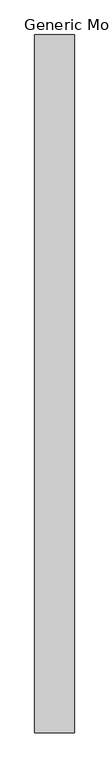
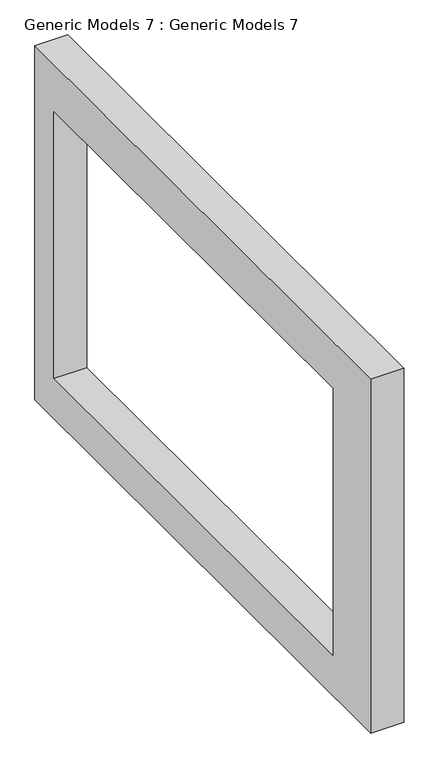
"""IFC4 building model written with IfcOpenShell, lengths in millimetres: proxy geometry, Generic Models 7 : Generic Models 7."""

from ifc_helpers import new_model, si_unit, frame, origin, place, context, project, spatial, polyline, outline, extrude, source, transform, mapped, element, save


def generic_models_7_generic_models_7_aecf1bf8(model_context):
    return source(origin(), model_context, "Body", "SweptSolid", [
        extrude(outline(polyline([(-2268.3844117, 3048.0), (-7640.6478449, 3048.0), (-7640.6478449, 6502.4), (-2268.3844117, 6502.4), (-2268.3844117, 3048.0)]), holes=[polyline([(-2573.1844117, 6045.2), (-7030.8844117, 6045.2), (-7030.8844117, 3438.5940938), (-2573.1844117, 3438.5940938), (-2573.1844117, 6045.2)])]), frame((66.1413992, 0.0, 0.0), z_axis=(1.0, 0.0, 0.0), x_axis=(0.0, 1.0, 0.0)), (0.0, 0.0, 1.0), 304.8),
    ])


if __name__ == "__main__":
    model = new_model("IFC4")
    model_context = context("Model", 3, world=origin())
    ifc_project = project(units=[si_unit("LENGTHUNIT", "METRE", prefix="MILLI")], contexts=[model_context])
    site = spatial("IfcSite", under=ifc_project)
    building = spatial("IfcBuilding", under=site)
    placement = place(None, origin())
    generic_models_7_generic_models_7_shape = generic_models_7_generic_models_7_aecf1bf8(model_context)
    element("IfcBuildingElementProxy", 1, Name="Generic Models 7 : Generic Models 7", ObjectType="Generic Models 7 : Generic Models 7", at=placement, inside=building, context=model_context, shape_type="MappedRepresentation", body=[
        mapped(generic_models_7_generic_models_7_shape, transform((0.0, 0.0, 0.0), x_axis=(1.0, 0.0, 0.0), y_axis=(0.0, 1.0, 0.0), z_axis=(0.0, 0.0, 1.0))),
    ])
    save(model, "model.ifc")

# Revit data of these elements
# Element 1 (IfcBuildingElementProxy, "Generic Models 7 : Generic Models 7")
#   Materials on its faces: "feature frame"
# Materials
#   "feature frame": class "Generic", colour RGB 120 120 120, transparency 0, Cost = 0
